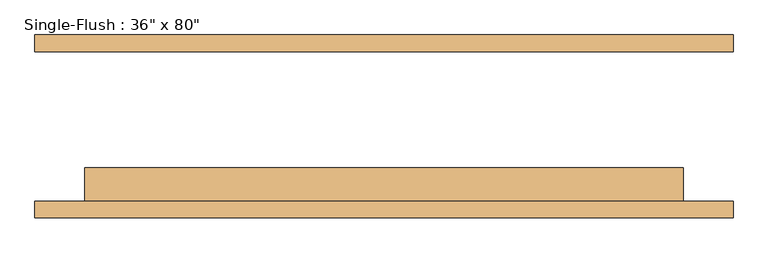
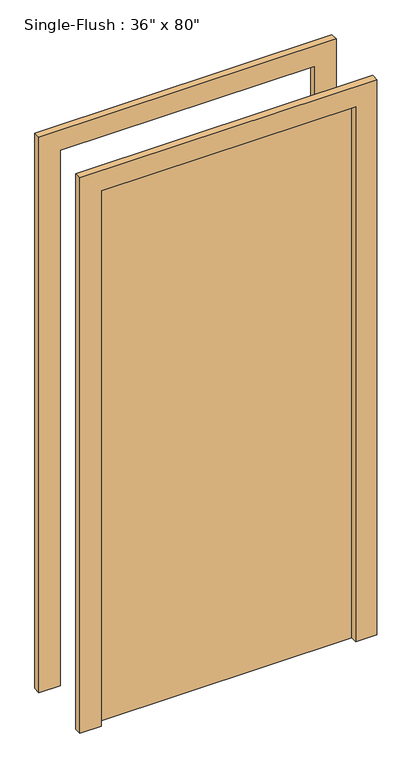
"""IFC4 building model written with IfcOpenShell, lengths in millimetres: door geometry."""

from ifc_helpers import new_model, si_unit, frame, origin, origin_with_axes, place, context, project, spatial, polyline, outline, extrude, source, transform, mapped, element, save


def door_ef0d591a(model_context):
    return source(origin(), model_context, "Body", "SweptSolid", [
        extrude(outline(polyline([(2108.2, -533.4), (0.0, -533.4), (0.0, -457.2), (2032.0, -457.2), (2032.0, 457.2), (0.0, 457.2), (0.0, 533.4), (2108.2, 533.4), (2108.2, -533.4)])), frame((0.0, -139.7, 0.0), z_axis=(0.0, 1.0, 0.0), x_axis=(0.0, 0.0, 1.0)), (0.0, 0.0, 1.0), 25.4),
        extrude(outline(polyline([(2108.2, 533.4), (2108.2, -533.4), (0.0, -533.4), (0.0, -457.2), (2032.0, -457.2), (2032.0, 457.2), (0.0, 457.2), (0.0, 533.4), (2108.2, 533.4)])), frame((0.0, 114.3, 0.0), z_axis=(0.0, 1.0, 0.0), x_axis=(0.0, 0.0, 1.0)), (0.0, 0.0, 1.0), 25.4),
        extrude(outline(polyline([(457.2, -63.5), (457.2, -114.3), (-457.2, -114.3), (-457.2, -63.5), (457.2, -63.5)])), origin_with_axes(), (0.0, 0.0, 1.0), 2032.0),
    ])


if __name__ == "__main__":
    model = new_model("IFC4")
    model_context = context("Model", 3, world=origin())
    ifc_project = project(units=[si_unit("LENGTHUNIT", "METRE", prefix="MILLI")], contexts=[model_context])
    site = spatial("IfcSite", under=ifc_project)
    building = spatial("IfcBuilding", under=site)
    placement = place(None, origin())
    door_shape = door_ef0d591a(model_context)
    element("IfcDoor", 1, ObjectType="Single-Flush : 36\" x 80\"", at=placement, inside=building, context=model_context, shape_type="MappedRepresentation", body=[
        mapped(door_shape, transform((0.0, 0.0, 0.0), x_axis=(1.0, 0.0, 0.0), y_axis=(0.0, 1.0, 0.0), z_axis=(0.0, 0.0, 1.0))),
    ])
    save(model, "model.ifc")

# Revit data of these elements
# Type "Single-Flush : 36\" x 80\""
#   Type Mark = "6"
#   Construction Type Id = "MDOOR"
#   Assembly Code = "C1020"
#   Analytic Construction = "Metal"
#   Thickness = 0' - 2"
#   Heat Transfer Coefficient (U) = 0.651978 BTU/(h·ft²·°F)
#   Height = 6' - 8"
#   Trim Projection Ext = 0' - 1"
#   Trim Projection Int = 0' - 1"
#   Trim Width = 0' - 3"
#   Width = 3' - 0"
#   Define Thermal Properties by = 1
#   Define Thermal Properties by = 1
#   Door Material = Door - Panel
#   Frame Material = Door - Frame
#   Visual Light Transmittance = 0
#   Solar Heat Gain Coefficient = 0
#   Function = (empty or 0)
#   Wall Closure = (empty or 0)
# Element 1 (IfcDoor, "Single-Flush : 36\" x 80\"")
#   Materials on its faces: "Door - Frame", "Door - Panel"
# Materials
#   "Door - Panel": class "Wood", colour RGB 210 159 95, transparency 0, Cost = 0
#   "Door - Frame": colour RGB 118 70 51, transparency 0, Cost = 0
